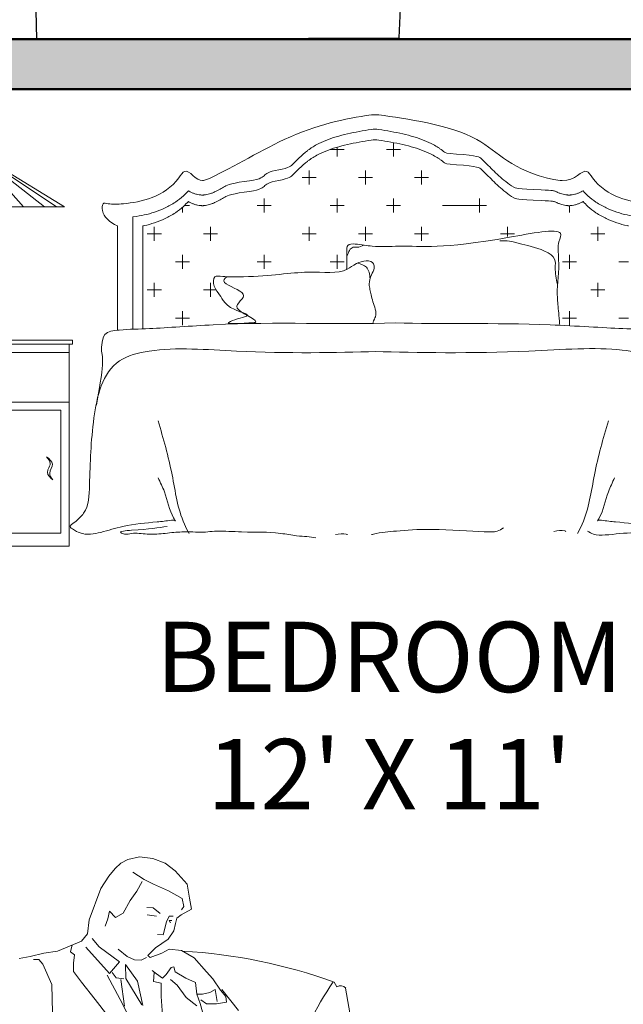
# Model space of a CAD drawing. Units: inches. Extents: x 1771 to 3025, y 319 to 889.
# Tile 28 of 35: x 2921 to 2982, y 521 to 619. Entities that reach past the tile are written whole.
import ezdxf

# ---------------------------------------------------------------- set-up
doc = ezdxf.new("R2010")
doc.units = ezdxf.units.IN
doc.header["$MEASUREMENT"] = 0
for name, color, linetype, lineweight in [('A-AREA-IDEN', 241, 'Continuous', 25), ('A-DOOR', 4, 'Continuous', 25), ('A-FURN', 8, 'Continuous', 18), ('A-WALL', 7, 'Continuous', 50), ('A-WALL-PATT', 254, 'Continuous', 13)]:
    doc.layers.add(name, color=color, linetype=linetype, lineweight=lineweight)
doc.styles.get("Standard").update_dxf_attribs({"font": 'arial.ttf'})

# ---------------------------------------------------------------- blocks, each defined once
blk = doc.blocks.new('A$C3908634B')
at = {"ltscale": 5}
for p, q in [((1200.2, 1046.3), (1218.1, 1046.3)), ((1176, 731), (1176, 731.7))]:
    blk.add_line(p, q, dxfattribs=at)
for p, q in [((1100.9, 962.2), (1134.6, 962.2)), ((1117.6, 945.1), (1117.6, 967.5)), ((1236.9, 962.2), (1271, 962.2)), ((1253.9, 945.1), (1253.9, 978.5)), ((266, 923.4), (356.4, 823.1)), ((278.7, 923.4), (406.8, 823.1)), ((284.7, 923.4), (436.3, 823.1)), ((290.6, 923.4), (456, 823.1)), ((1049.4, 876.9), (1049.4, 911)), ((1185.7, 876.9), (1185.7, 911)), ((1322.1, 876.9), (1322.1, 911)), ((1032.3, 894), (1066.4, 894)), ((1168.7, 894), (1202.8, 894)), ((1305.1, 894), (1339.1, 894)), ((940, 808.8), (940, 842.9)), ((1117.6, 808.8), (1117.6, 842.9)), ((1253.9, 808.8), (1253.9, 842.9)), ((1462.5, 808.8), (1462.5, 842.9)), ((237.5, 823.1), (456, 823.1)), ((741.7, 808.8), (741.7, 821.7)), ((746.2, 825.8), (758.8, 825.8)), ((922.9, 825.8), (957, 825.8)), ((1100.5, 825.8), (1134.6, 825.8)), ((1236.9, 825.8), (1271, 825.8)), ((1373.2, 825.8), (1479.5, 825.8)), ((1681.3, 808.8), (1681.3, 825.6)), ((621.3, 798.8), (621.3, 526)), ((645.8, 776.5), (645.8, 527)), ((673.5, 740.6), (673.5, 774.7)), ((809.9, 740.6), (809.9, 774.7)), ((1049.4, 740.6), (1049.4, 774.7)), ((1185.7, 740.6), (1185.7, 774.7)), ((1322.1, 740.6), (1322.1, 774.7)), ((1530.6, 751.3), (1530.6, 774.7)), ((1749.5, 740.6), (1749.5, 774.7)), ((656.5, 757.6), (690.6, 757.6)), ((792.9, 757.6), (827, 757.6)), ((1032.3, 757.6), (1066.4, 757.6)), ((1168.7, 757.6), (1202.8, 757.6)), ((1305.1, 757.6), (1339.1, 757.6)), ((1513.6, 757.6), (1547.7, 757.6)), ((1732.4, 757.6), (1766.5, 757.6)), ((741.7, 672.4), (741.7, 706.5)), ((940, 672.4), (940, 706.5)), ((1117.6, 672.4), (1117.6, 706.5)), ((1681.3, 672.4), (1681.3, 706.5)), ((724.7, 689.4), (758.8, 689.4)), ((922.9, 689.4), (957, 689.4)), ((1100.5, 689.4), (1134.6, 689.4)), ((1664.3, 689.4), (1698.3, 689.4)), ((1800.6, 689.4), (1824, 689.4)), ((656.5, 621.3), (690.6, 621.3)), ((673.5, 604.2), (673.5, 638.3)), ((792.9, 621.3), (823.2, 621.3)), ((809.9, 604.2), (809.9, 638.3)), ((1732.4, 621.3), (1766.5, 621.3)), ((1749.5, 604.2), (1749.5, 638.3)), ((724.7, 553.1), (758.8, 553.1)), ((741.7, 536), (741.7, 570.1)), ((1664.3, 553.1), (1698.3, 553.1)), ((1681.3, 536), (1681.3, 570.1)), ((1800.6, 553.1), (1824, 553.1)), ((475, 499.5), (0, 499.5)), ((475, 489.5), (0, 489.5)), ((467.1, 0), (467.1, 489.5)), ((475, 499.5), (475, 489.5)), ((467.1, 469.5), (8.7, 469.5)), ((467.1, 349.5), (8.7, 349.5)), ((447.1, 329.5), (28.7, 329.5)), ((447.1, 31.6), (447.1, 329.5)), ((467.1, 281.6), (467.1, 301.6)), ((28.7, 31.6), (447.1, 31.6)), ((8.7, 0), (467.1, 0))]:
    blk.add_line(p, q)
at = {"ltscale": 20}
blk.add_line((584.4, 776.7), (584.4, 523.7), dxfattribs=at)
for centre in [(1209.1, 956.2), (1209.1, 930.3)]:
    blk.add_arc(centre, 55.2, 80.5605, 99.4395)
for points in [[(584.4, 776.7), (563.9, 786.2), (546, 802.1), (547.3, 834.8), (564.5, 828.3), (620.6, 830.4), (706.4, 847.2), (752.1, 924.2), (778.1, 880.4), (846.1, 907.1), (1017.7, 1014.1), (1134.5, 1035.5), (1200.2, 1046.3)], [(1885.4, 776.7), (1905.9, 786.2), (1923.9, 802.1), (1922.5, 834.8), (1905.3, 828.3), (1849.2, 830.4), (1763.4, 847.2), (1717.7, 924.2), (1691.7, 880.4), (1541.2, 907.1), (1472.8, 1014.1), (1283.8, 1035.5), (1218.1, 1046.3)]]:
    blk.add_open_spline(points, degree=3, knots=[12.417853, 12.417853, 12.417853, 12.417853, 68.394536, 90.665986, 114.156853, 157.554067, 281.869614, 298.858744, 338.737111, 347.060176, 470.423438, 625.498764, 625.498764, 625.498764, 625.498764], dxfattribs=at)
for points, knots in [([(756.1, 861.8), (756.9, 861.3), (757.6, 860.9), (759.9, 859.6), (761.6, 858.7), (765.5, 856.8), (767.8, 855.8), (772.7, 854.1), (775.4, 853.3), (780.8, 852.2), (783.3, 851.8), (787.1, 851.6), (788.2, 851.5), (789.9, 851.5), (790.6, 851.5), (791.9, 851.5), (792.5, 851.5), (793.6, 851.6), (794.1, 851.6), (795.8, 851.8), (796.8, 851.9), (800.3, 852.3), (802.5, 852.8), (806.5, 853.8), (808.3, 854.3), (811.5, 855.4), (812.9, 855.9), (815.3, 856.9), (816.4, 857.4), (817.6, 857.9), (817.8, 858), (818.4, 858.2), (818.7, 858.4), (819.5, 858.7), (820, 859), (821.6, 859.7), (822.7, 860.2), (825.8, 861.7), (827.9, 862.8), (834, 866), (837.9, 868.3), (848.5, 874.9), (854.9, 879.4), (928.8, 888.8), (934.4, 893.5), (945, 903.2), (950, 908), (1000.9, 917.4), (1005.5, 922.1), (1014.4, 931), (1018.7, 935.3), (1027, 943.5), (1031.1, 947.3), (1036.9, 952.4), (1038.8, 954), (1042, 956.7), (1043.5, 957.9), (1045.8, 959.7), (1046.7, 960.3), (1048.5, 961.7), (1049.4, 962.3), (1052.1, 964.2), (1054, 965.5), (1059.7, 969.2), (1063.6, 971.5), (1074.8, 977.5), (1082.2, 980.9), (1098, 987.2), (1106.3, 990), (1123.7, 995.2), (1132.8, 997.5), (1151.5, 1001.8), (1161.1, 1003.8), (1180.5, 1007.4), (1190.2, 1009), (1200.1, 1010.7)], [328.6705, 328.6705, 328.6705, 328.6705, 329.609368, 329.609368, 331.487103, 331.487103, 333.620342, 333.620342, 335.753581, 335.753581, 337.507866, 337.507866, 338.182373, 338.182373, 338.607397, 338.607397, 338.959312, 338.959312, 339.311227, 339.311227, 340.015058, 340.015058, 341.722742, 341.722742, 343.430427, 343.430427, 345.138111, 345.138111, 346.845796, 346.845796, 347.37881, 347.37881, 347.911824, 347.911824, 348.977853, 348.977853, 351.109909, 351.109909, 355.374023, 355.374023, 363.902249, 363.902249, 379.258481, 379.258481, 394.614712, 394.614712, 409.970944, 409.970944, 425.327175, 425.327175, 440.683406, 440.683406, 456.039638, 456.039638, 463.285514, 463.285514, 469.01116, 469.01116, 472.593, 472.593, 476.17484, 476.17484, 483.338521, 483.338521, 497.665882, 497.665882, 522.309302, 522.309302, 546.952723, 546.952723, 571.596143, 571.596143, 596.239564, 596.239564, 619.876409, 619.876409, 619.876409, 619.876409]), ([(1713.7, 861.8), (1713, 861.3), (1712.2, 860.9), (1709.9, 859.6), (1708.2, 858.7), (1704.3, 856.8), (1702.1, 855.8), (1697.1, 854.1), (1694.4, 853.3), (1689.1, 852.2), (1686.5, 851.8), (1682.7, 851.6), (1681.7, 851.5), (1679.9, 851.5), (1679.2, 851.5), (1678, 851.5), (1677.4, 851.5), (1676.2, 851.6), (1675.7, 851.6), (1674.1, 851.8), (1673, 851.9), (1669.5, 852.3), (1667.3, 852.8), (1663.3, 853.8), (1661.5, 854.3), (1658.4, 855.4), (1657, 855.9), (1654.5, 856.9), (1653.4, 857.4), (1652.2, 857.9), (1652, 858), (1651.4, 858.2), (1651.2, 858.4), (1650.4, 858.7), (1649.8, 859), (1648.2, 859.7), (1647.1, 860.2), (1644, 861.7), (1641.9, 862.8), (1553.3, 866), (1549.4, 868.3), (1538.8, 874.9), (1532.4, 879.4), (1520.4, 888.8), (1514.8, 893.5), (1504.2, 903.2), (1499.2, 908), (1489.5, 917.4), (1484.9, 922.1), (1476.1, 931), (1471.8, 935.3), (1463.4, 943.5), (1459.4, 947.3), (1381.4, 952.4), (1379.5, 954), (1376.2, 956.7), (1374.8, 957.9), (1372.5, 959.7), (1371.6, 960.3), (1369.8, 961.7), (1368.9, 962.3), (1366.2, 964.2), (1364.3, 965.5), (1358.6, 969.2), (1354.6, 971.5), (1343.5, 977.5), (1336, 980.9), (1320.2, 987.2), (1311.9, 990), (1294.6, 995.2), (1285.5, 997.5), (1266.8, 1001.8), (1257.2, 1003.8), (1237.8, 1007.4), (1228.1, 1009), (1218.2, 1010.7)], [328.6705, 328.6705, 328.6705, 328.6705, 329.609368, 329.609368, 331.487103, 331.487103, 333.620342, 333.620342, 335.753581, 335.753581, 337.507866, 337.507866, 338.182373, 338.182373, 338.607397, 338.607397, 338.959312, 338.959312, 339.311227, 339.311227, 340.015058, 340.015058, 341.722742, 341.722742, 343.430427, 343.430427, 345.138111, 345.138111, 346.845796, 346.845796, 347.37881, 347.37881, 347.911824, 347.911824, 348.977853, 348.977853, 351.109909, 351.109909, 355.374023, 355.374023, 363.902249, 363.902249, 379.258481, 379.258481, 394.614712, 394.614712, 409.970943, 409.970943, 425.327175, 425.327175, 440.683406, 440.683406, 456.039637, 456.039637, 463.285514, 463.285514, 469.011154, 469.011154, 472.592992, 472.592992, 476.17483, 476.17483, 483.338506, 483.338506, 497.665857, 497.665857, 522.309275, 522.309275, 546.952693, 546.952693, 571.59611, 571.59611, 596.239528, 596.239528, 619.876409, 619.876409, 619.876409, 619.876409]), ([(756.1, 835.9), (756.9, 835.5), (757.6, 835), (759.9, 833.7), (761.6, 832.8), (765.5, 830.9), (767.8, 830), (772.7, 828.2), (775.4, 827.5), (780.8, 826.3), (783.3, 826), (787.1, 825.7), (788.2, 825.7), (789.9, 825.6), (790.6, 825.6), (791.9, 825.6), (792.5, 825.7), (793.6, 825.7), (794.1, 825.8), (795.8, 825.9), (796.8, 826), (800.3, 826.5), (802.5, 826.9), (806.5, 827.9), (808.3, 828.5), (811.5, 829.5), (812.9, 830.1), (815.3, 831), (816.4, 831.5), (817.6, 832), (817.8, 832.1), (818.4, 832.4), (818.7, 832.5), (819.5, 832.9), (820, 833.1), (821.6, 833.8), (822.7, 834.3), (825.8, 835.9), (827.9, 836.9), (834, 840.2), (837.9, 842.4), (848.5, 849), (854.9, 853.6), (928.8, 862.9), (934.4, 867.7), (945, 877.3), (950, 882.1), (1000.9, 891.6), (1005.5, 896.2), (1014.4, 905.2), (1018.7, 909.5), (1027, 917.6), (1031.1, 921.4), (1036.9, 926.6), (1038.8, 928.2), (1042, 930.9), (1043.5, 932), (1045.8, 933.8), (1046.7, 934.5), (1048.5, 935.8), (1049.4, 936.4), (1052.1, 938.4), (1054, 939.6), (1059.7, 943.3), (1063.6, 945.6), (1074.8, 951.6), (1082.2, 955), (1098, 961.3), (1106.3, 964.2), (1123.7, 969.3), (1132.8, 971.6), (1151.5, 975.9), (1161.1, 977.9), (1180.5, 981.5), (1190.2, 983.2), (1200.1, 984.8)], [328.6705, 328.6705, 328.6705, 328.6705, 329.609368, 329.609368, 331.487103, 331.487103, 333.620342, 333.620342, 335.753581, 335.753581, 337.507866, 337.507866, 338.182373, 338.182373, 338.607397, 338.607397, 338.959312, 338.959312, 339.311227, 339.311227, 340.015058, 340.015058, 341.722742, 341.722742, 343.430427, 343.430427, 345.138111, 345.138111, 346.845796, 346.845796, 347.37881, 347.37881, 347.911824, 347.911824, 348.977853, 348.977853, 351.109909, 351.109909, 355.374023, 355.374023, 363.902249, 363.902249, 379.258481, 379.258481, 394.614712, 394.614712, 409.970944, 409.970944, 425.327175, 425.327175, 440.683406, 440.683406, 456.039638, 456.039638, 463.285514, 463.285514, 469.01116, 469.01116, 472.593, 472.593, 476.17484, 476.17484, 483.338521, 483.338521, 497.665882, 497.665882, 522.309302, 522.309302, 546.952723, 546.952723, 571.596143, 571.596143, 596.239564, 596.239564, 619.876409, 619.876409, 619.876409, 619.876409]), ([(1713.7, 835.9), (1713, 835.5), (1712.2, 835), (1709.9, 833.7), (1708.2, 832.8), (1704.3, 830.9), (1702.1, 830), (1697.1, 828.2), (1694.4, 827.5), (1689.1, 826.3), (1686.5, 826), (1682.7, 825.7), (1681.7, 825.7), (1679.9, 825.6), (1679.2, 825.6), (1678, 825.6), (1677.4, 825.7), (1676.2, 825.7), (1675.7, 825.8), (1674.1, 825.9), (1673, 826), (1669.5, 826.5), (1667.3, 826.9), (1663.3, 827.9), (1661.5, 828.5), (1658.4, 829.5), (1657, 830.1), (1654.5, 831), (1653.4, 831.5), (1652.2, 832), (1652, 832.1), (1651.4, 832.4), (1651.2, 832.5), (1650.4, 832.9), (1649.8, 833.1), (1648.2, 833.8), (1647.1, 834.3), (1644, 835.9), (1641.9, 836.9), (1553.3, 840.2), (1549.4, 842.4), (1538.8, 849), (1532.4, 853.6), (1520.4, 862.9), (1514.8, 867.7), (1504.2, 877.3), (1499.2, 882.1), (1489.5, 891.6), (1484.9, 896.2), (1476.1, 905.2), (1471.8, 909.5), (1463.4, 917.6), (1459.4, 921.4), (1381.4, 926.6), (1379.5, 928.2), (1376.2, 930.9), (1374.8, 932), (1372.5, 933.8), (1371.6, 934.5), (1369.8, 935.8), (1368.9, 936.4), (1366.2, 938.4), (1364.3, 939.6), (1358.6, 943.3), (1354.6, 945.6), (1343.5, 951.6), (1336, 955), (1320.2, 961.3), (1311.9, 964.2), (1294.6, 969.3), (1285.5, 971.6), (1266.8, 975.9), (1257.2, 977.9), (1237.8, 981.5), (1228.1, 983.2), (1218.2, 984.8)], [328.6705, 328.6705, 328.6705, 328.6705, 329.609368, 329.609368, 331.487103, 331.487103, 333.620342, 333.620342, 335.753581, 335.753581, 337.507866, 337.507866, 338.182373, 338.182373, 338.607397, 338.607397, 338.959312, 338.959312, 339.311227, 339.311227, 340.015058, 340.015058, 341.722742, 341.722742, 343.430427, 343.430427, 345.138111, 345.138111, 346.845796, 346.845796, 347.37881, 347.37881, 347.911824, 347.911824, 348.977853, 348.977853, 351.109909, 351.109909, 355.374023, 355.374023, 363.902249, 363.902249, 379.258481, 379.258481, 394.614712, 394.614712, 409.970943, 409.970943, 425.327175, 425.327175, 440.683406, 440.683406, 456.039637, 456.039637, 463.285514, 463.285514, 469.011154, 469.011154, 472.592992, 472.592992, 476.17483, 476.17483, 483.338506, 483.338506, 497.665857, 497.665857, 522.309275, 522.309275, 546.952693, 546.952693, 571.59611, 571.59611, 596.239528, 596.239528, 619.876409, 619.876409, 619.876409, 619.876409]), ([(621.3, 798.8), (633.4, 799.9), (641.2, 801.3), (657.3, 805), (665.7, 807.2), (682.6, 812.8), (691.1, 816.1), (708.1, 824.2), (716.5, 828.9), (731.3, 839), (737.9, 844.1), (748.3, 853.5), (752.3, 857.5), (756.1, 861.8)], [179.330708, 179.330708, 179.330708, 179.330708, 196.086144, 196.086144, 213.445516, 213.445516, 230.804888, 230.804888, 248.16426, 248.16426, 262.451931, 262.451931, 271.832526, 271.832526, 271.832526, 271.832526]), ([(1848.6, 798.8), (1836.4, 799.9), (1828.6, 801.3), (1812.5, 805), (1804.1, 807.2), (1787.2, 812.8), (1778.7, 816.1), (1761.8, 824.2), (1753.4, 828.9), (1738.5, 839), (1731.9, 844.1), (1721.5, 853.5), (1717.5, 857.5), (1713.7, 861.8)], [179.400376, 179.400376, 179.400376, 179.400376, 196.086144, 196.086144, 213.445516, 213.445516, 230.804888, 230.804888, 248.16426, 248.16426, 262.451931, 262.451931, 271.832526, 271.832526, 271.832526, 271.832526]), ([(645.8, 776.5), (646.9, 776.7), (648, 777), (657.3, 779.1), (665.7, 781.3), (682.6, 786.9), (691.1, 790.3), (708.1, 798.3), (716.5, 803), (731.3, 813.1), (737.9, 818.2), (748.3, 827.7), (752.3, 831.7), (756.1, 835.9)], [193.740688, 193.740688, 193.740688, 193.740688, 196.086144, 196.086144, 213.445516, 213.445516, 230.804888, 230.804888, 248.16426, 248.16426, 262.451931, 262.451931, 271.832526, 271.832526, 271.832526, 271.832526]), ([(1824, 776.5), (1822.9, 776.7), (1821.8, 777), (1812.5, 779.1), (1804.1, 781.3), (1787.2, 786.9), (1778.7, 790.3), (1761.8, 798.3), (1753.4, 803), (1738.5, 813.1), (1731.9, 818.2), (1721.5, 827.7), (1717.5, 831.7), (1713.7, 835.9)], [193.740688, 193.740688, 193.740688, 193.740688, 196.086144, 196.086144, 213.445516, 213.445516, 230.804888, 230.804888, 248.16426, 248.16426, 262.451931, 262.451931, 271.832526, 271.832526, 271.832526, 271.832526]), ([(1512.2, 740.7), (1519.9, 740.7), (1533.1, 740.8), (1553.9, 735.5), (1652.4, 710.7), (1643.1, 675.3), (1648.8, 648.1), (1651.8, 634.5), (1651.9, 634)], [0, 0, 0, 0, 31.268494, 53.71641, 83.24833, 138.583941, 192.96698, 194.695488, 194.695488, 194.695488, 194.695488]), ([(1181.8, 730.2), (1176.9, 727.3), (1167.9, 723.5), (1152.3, 726.4), (1145.2, 713.6), (1142.1, 705.5), (1140.6, 701.2)], [16.588235, 16.588235, 16.588235, 16.588235, 39.368234, 56.465167, 72.647278, 91.317886, 91.317886, 91.317886, 91.317886]), ([(1167.2, 686.5), (1175.5, 684.3), (1192.8, 677.8), (1196.3, 659.6), (1197.1, 648.3)], [13.535772, 13.535772, 13.535772, 13.535772, 45.871957, 87.312392, 87.312392, 87.312392, 87.312392]), ([(849.2, 653.1), (844.3, 648.8), (832.7, 636.7), (919.4, 609.9), (841.8, 577.9), (927.1, 550.1), (918.1, 541), (854.7, 539.8)], [5.952535, 5.952535, 5.952535, 5.952535, 29.258845, 70.114919, 115.518645, 162.322231, 169.813565, 169.813565, 169.813565, 169.813565]), ([(412.3, 216.6), (419.2, 211), (432.8, 199.9), (414.9, 178.1), (423.4, 166), (427.2, 160.5)], [0, 0, 0, 0, 22.772447, 45.052082, 63.466582, 63.466582, 63.466582, 63.466582]), ([(412.3, 216.6), (416.7, 211.4), (424.6, 201.9), (416.9, 189), (411.8, 174.1), (420.6, 166.3), (427.2, 160.5)], [0, 0, 0, 0, 18.381528, 32.980054, 40.875646, 63.595153, 63.595153, 63.595153, 63.595153])]:
    blk.add_open_spline(points, degree=3, knots=knots)
at = {"ltscale": 5}
for points, knots in [([(1140.2, 671), (1140.5, 684.2), (1141, 702.6), (1139.6, 733.3), (1171.5, 732.8), (1207.8, 724.4), (1313, 731.7), (1377.9, 716.1), (1675.3, 776), (1653.6, 739.3), (1653.4, 708.6), (1656.7, 669.4), (1649.8, 624.8), (1652.8, 584.9), (1655.4, 559.2), (1656.8, 538.3)], [3.603347, 3.603347, 3.603347, 3.603347, 60.838375, 82.182907, 107.012175, 163.177093, 249.239778, 501.114283, 577.787612, 607.274607, 630.949286, 706.159707, 762.92633, 812.910096, 867.096105, 867.096105, 867.096105, 867.096105]), ([(853.1, 539.8), (853.8, 547.4), (919.3, 558.2), (845.3, 575.8), (836.7, 609.7), (818, 623.2), (814.4, 657.6), (840.5, 653), (943.6, 652.6), (1051.1, 671.7), (1127.7, 657.4), (1165, 689.4), (1205, 697), (1208.2, 671.1), (1198.6, 657.5), (1193.8, 634.4), (1197.9, 619.2), (1201.2, 597.1), (1215.4, 563.6), (1206.8, 549.2), (1203.5, 540.2)], [33.020195, 33.020195, 33.020195, 33.020195, 57.294753, 90.473933, 194.149416, 257.058105, 304.592565, 338.383824, 389.043604, 577.649845, 759.359611, 813.032269, 898.973184, 920.659088, 956.429806, 1000.911745, 1042.797508, 1121.842246, 1191.460876, 1213.109701, 1213.109701, 1213.109701, 1213.109701]), ([(533.2, 342.2), (554.6, 456.3), (543.3, 464.8), (546.8, 491.4), (549.9, 520.4), (602.8, 525.9), (675.3, 527.2), (929.2, 547.1), (1113.3, 536.9), (1259.7, 541.4)], [0, 0, 0, 0, 32.681627, 48.455722, 75.25348, 112.004017, 183.381957, 310.642358, 688.088714, 688.088714, 688.088714, 688.088714]), ([(1911, 390.4), (1911.9, 458.8), (1930, 464.8), (1926.5, 491.4), (1923.4, 520.4), (1870.5, 525.9), (1798, 527.2), (1556.5, 543.7), (1364.8, 538.4), (1259.7, 541.4)], [0, 0, 0, 0, 32.681627, 48.455722, 75.25348, 112.004017, 183.381957, 310.642358, 588.939547, 588.939547, 588.939547, 588.939547]), ([(482.8, 59.4), (489.8, 65.8), (514.7, 88.6), (517.4, 182.5), (520.5, 297.5), (551.9, 447.1), (697, 485.5), (926.3, 465.8), (1116.6, 468.9), (1210.9, 472.2)], [0, 0, 0, 0, 28.320233, 100.953775, 269.820348, 420.691469, 489.161544, 656.134073, 940.569207, 940.569207, 940.569207, 940.569207]), ([(1990.5, 59.4), (1983.5, 65.8), (1958.6, 88.6), (1942.6, 182.5), (1920.4, 297.5), (1912.1, 455.6), (1776.3, 485.5), (1526.4, 465.8), (1305.2, 468.9), (1210.9, 472.2)], [0, 0, 0, 0, 28.320233, 100.953775, 269.820348, 420.691469, 489.161544, 656.134073, 940.569207, 940.569207, 940.569207, 940.569207]), ([(682.9, 304.1), (695.4, 260.8), (719.1, 178.1), (730.8, 82.2), (753.9, 38.3), (757.8, 30.9)], [0, 0, 0, 0, 135.247847, 258.692787, 283.800228, 283.800228, 283.800228, 283.800228]), ([(1775.2, 304.1), (1762.7, 260.8), (1739, 178.1), (1727.3, 82.2), (1704.2, 38.3), (1700.3, 30.9)], [0, 0, 0, 0, 135.247847, 258.692787, 283.800228, 283.800228, 283.800228, 283.800228]), ([(682.9, 165.6), (688.3, 154.5), (703.5, 123.2), (710.2, 85), (723.1, 63.5), (724.6, 61.1)], [0, 0, 0, 0, 37.234018, 105.386078, 113.844905, 113.844905, 113.844905, 113.844905]), ([(1790.4, 165.6), (1785, 154.5), (1769.8, 123.2), (1763.1, 85), (1750.2, 63.5), (1748.7, 61.1)], [0, 0, 0, 0, 37.234018, 105.386078, 113.844905, 113.844905, 113.844905, 113.844905]), ([(482.8, 59.4), (474.7, 54.3), (464, 47.4), (477.3, 41.4), (486.1, 33.4), (496.5, 31.3), (502.9, 30)], [0, 0, 0, 0, 19.035414, 25.269998, 36.960672, 56.00812, 56.00812, 56.00812, 56.00812]), ([(504.2, 28.9), (509, 28.7), (522.4, 28.3), (553.7, 35.4), (605.7, 52.4), (665.1, 57), (705.3, 61.4), (721.5, 63.6), (724.2, 61.4), (724.6, 61.1)], [0, 0, 0, 0, 14.447875, 40.468341, 96.220884, 181.018327, 216.046098, 224.609189, 226.185962, 226.185962, 226.185962, 226.185962]), ([(1969.1, 28.9), (1964.3, 28.7), (1950.9, 28.3), (1919.6, 35.4), (1867.6, 52.4), (1808.2, 57), (1768, 61.4), (1751.8, 63.6), (1749.1, 61.4), (1748.7, 61.1)], [0, 0, 0, 0, 14.447875, 40.468341, 96.220884, 181.018327, 216.046098, 224.609189, 226.185962, 226.185962, 226.185962, 226.185962]), ([(704.5, 47.7), (683.7, 44.6), (656.6, 40.6), (582.3, 36), (604.8, 26.7), (618.5, 32.3), (643.5, 30.4), (675.7, 27.4), (715, 33.3), (758.1, 35.6), (793.8, 32.4), (824.3, 37.8), (918.5, 32.1), (952.2, 36.4), (1023, 23.8), (1044.1, 24.1), (1058.3, 21.3), (1065.7, 20.4)], [0, 0, 0, 0, 87.513803, 114.592793, 124.77702, 141.903576, 160.817021, 198.691115, 240.471478, 280.23486, 329.410006, 348.41762, 373.077233, 428.05708, 447.802257, 468.691939, 491.310217, 491.310217, 491.310217, 491.310217]), ([(1113.3, 28), (1122.2, 29.4), (1132.2, 31.9), (1141.4, 28.4), (1142.4, 28)], [516.212662, 516.212662, 516.212662, 516.212662, 542.681017, 546.007116, 546.007116, 546.007116, 546.007116]), ([(1200.5, 28), (1202, 28.4), (1222.7, 33.5), (1266.3, 36.8), (1334.2, 43.2), (1462.5, 35), (1502.7, 33.5), (1515.8, 41.2), (1520.7, 44.1)], [590.079786, 590.079786, 590.079786, 590.079786, 594.646549, 651.888327, 725.747367, 797.841373, 826.274406, 843.189267, 843.189267, 843.189267, 843.189267]), ([(1643.2, 35.6), (1652.1, 37), (1662.2, 39.5), (1671.4, 36), (1672.4, 35.6)], [516.212662, 516.212662, 516.212662, 516.212662, 542.681017, 546.007116, 546.007116, 546.007116, 546.007116]), ([(1972.3, 20.4), (1970.7, 20.8), (1950, 25.9), (1906.5, 29.2), (1838.6, 35.6), (1782.4, 27.4), (1742.2, 25.9), (1729.1, 33.6), (1724.3, 36.5)], [590.079786, 590.079786, 590.079786, 590.079786, 594.646549, 651.888327, 725.747367, 797.841373, 826.274406, 843.189267, 843.189267, 843.189267, 843.189267])]:
    blk.add_open_spline(points, degree=3, knots=knots, dxfattribs=at)
blk = doc.blocks.new('A$C0DCF6C46')
for p, q in [((1202.6, 1072.4), (1213.4, 1083.3)), ((1202.6, 1072.4), (1213.4, 1083.3)), ((1213.4, 1083.3), (1227.6, 1090.4)), ((1213.4, 1083.3), (1227.6, 1090.4)), ((1227.6, 1090.4), (1251, 1095.4)), ((1227.6, 1090.4), (1251, 1095.4)), ((1251, 1095.4), (1277.5, 1092)), ((1251, 1095.4), (1277.5, 1092)), ((1277.5, 1092), (1301.8, 1082.8)), ((1277.5, 1092), (1301.8, 1082.8)), ((1301.8, 1082.8), (1321.9, 1067.8)), ((1301.8, 1082.8), (1321.9, 1067.8)), ((1173.6, 1032.9), (1189.7, 1057.2)), ((1173.6, 1032.9), (1189.7, 1057.2)), ((1189.7, 1057.2), (1202.6, 1072.4)), ((1189.7, 1057.2), (1202.6, 1072.4)), ((1259.7, 1050.3), (1237.5, 1065.3)), ((1259.7, 1050.3), (1237.5, 1065.3)), ((1321.9, 1067.8), (1345.5, 1041.1)), ((1321.9, 1067.8), (1345.5, 1041.1)), ((1255.9, 1046.6), (1245.7, 1027.6)), ((1255.9, 1046.6), (1245.7, 1027.6)), ((1278.7, 1041.6), (1259.7, 1050.3)), ((1278.7, 1041.6), (1259.7, 1050.3)), ((1308.3, 1028.1), (1278.7, 1041.6)), ((1308.3, 1028.1), (1278.7, 1041.6)), ((1345.5, 1041.1), (1350.1, 1013.5)), ((1345.5, 1041.1), (1350.1, 1013.5)), ((1150.8, 970.5), (1173.6, 1032.9)), ((1150.8, 970.5), (1173.6, 1032.9)), ((1245.7, 1027.6), (1232.3, 1009.1)), ((1245.7, 1027.6), (1232.3, 1009.1)), ((1335.8, 1012.5), (1308.3, 1028.1)), ((1335.8, 1012.5), (1308.3, 1028.1)), ((1232.3, 1009.1), (1218.3, 983.7)), ((1232.3, 1009.1), (1218.3, 983.7)), ((1338.8, 997.1), (1335.8, 1012.5)), ((1338.8, 997.1), (1335.8, 1012.5)), ((1350.1, 1013.5), (1354.2, 991.7)), ((1350.1, 1013.5), (1354.2, 991.7)), ((1190.8, 987.7), (1188, 972.3)), ((1190.8, 987.7), (1188, 972.3)), ((1202.9, 975.4), (1190.8, 987.7)), ((1202.9, 975.4), (1190.8, 987.7)), ((1218.3, 983.7), (1202.9, 975.4)), ((1218.3, 983.7), (1202.9, 975.4)), ((1277.8, 994.4), (1265.6, 995)), ((1277.8, 994.4), (1265.6, 995)), ((1266, 980.7), (1284.6, 977.9)), ((1266, 980.7), (1284.6, 977.9)), ((1291.5, 983.2), (1277.8, 994.4)), ((1291.5, 983.2), (1277.8, 994.4)), ((1333.4, 980.2), (1324.9, 973.9)), ((1333.4, 980.2), (1324.9, 973.9)), ((1354.2, 991.7), (1333.4, 980.2)), ((1354.2, 991.7), (1333.4, 980.2)), ((1334, 990.3), (1338.8, 997.1)), ((1334, 990.3), (1338.8, 997.1)), ((1147.4, 942.9), (1150.8, 970.5)), ((1147.4, 942.9), (1150.8, 970.5)), ((1188, 972.3), (1182.6, 958)), ((1188, 972.3), (1182.6, 958)), ((1304.1, 966.6), (1297.6, 940.6)), ((1304.1, 966.6), (1297.6, 940.6)), ((1309.5, 977.7), (1304.1, 966.6)), ((1309.5, 977.7), (1304.1, 966.6)), ((1309.4, 969), (1312.6, 964.7)), ((1314.7, 968.9), (1309.4, 969)), ((1309.4, 969), (1312.6, 964.7)), ((1314.7, 968.9), (1309.4, 969)), ((1317.5, 977.7), (1309.5, 977.7)), ((1317.5, 977.7), (1309.5, 977.7)), ((1322.1, 963.3), (1318.8, 948.5)), ((1322.1, 963.3), (1318.8, 948.5)), ((1324.9, 973.9), (1322.1, 963.3)), ((1324.9, 973.9), (1322.1, 963.3)), ((1135.7, 928.2), (1147.4, 942.9)), ((1135.7, 928.2), (1147.4, 942.9)), ((1297.6, 940.6), (1286.8, 941.4)), ((1297.6, 940.6), (1286.8, 941.4)), ((1318.8, 948.5), (1307.6, 932.1)), ((1318.8, 948.5), (1307.6, 932.1)), ((1087.8, 908.4), (1135.7, 928.2)), ((1087.8, 908.4), (1135.7, 928.2)), ((1117, 920.9), (1113.7, 907.1)), ((1117, 920.9), (1113.7, 907.1)), ((1170.4, 917.1), (1156.8, 933.1)), ((1170.4, 917.1), (1156.8, 933.1)), ((1307.6, 932.1), (1282.5, 914.8)), ((1307.6, 932.1), (1282.5, 914.8)), ((1033.6, 897.7), (1060.7, 904.4)), ((1033.6, 897.7), (1060.7, 904.4)), ((1060.7, 904.4), (1087.8, 908.4)), ((1060.7, 904.4), (1087.8, 908.4)), ((1113.7, 907.1), (1121.7, 900.7)), ((1113.7, 907.1), (1121.7, 900.7)), ((1121.7, 900.7), (1119.4, 884.3)), ((1121.7, 900.7), (1119.4, 884.3)), ((1190.9, 864.1), (1144, 915.9)), ((1190.9, 864.1), (1144, 915.9)), ((1211.2, 886.7), (1170.4, 917.1)), ((1211.2, 886.7), (1170.4, 917.1)), ((1225.9, 897.6), (1208.3, 912.3)), ((1225.9, 897.6), (1208.3, 912.3)), ((1282.5, 914.8), (1267, 899.5)), ((1282.5, 914.8), (1267, 899.5)), ((1271.7, 895.8), (1295.1, 904.1)), ((1271.7, 895.8), (1295.1, 904.1)), ((1295.1, 904.1), (1310, 911.9)), ((1295.1, 904.1), (1310, 911.9)), ((1310, 911.9), (1334.4, 909.6)), ((1310, 911.9), (1334.4, 909.6)), ((1334.4, 909.6), (1359.2, 894.6)), ((1334.4, 909.6), (1359.2, 894.6)), ((1011.8, 893.6), (1033.6, 897.7)), ((1011.8, 893.6), (1033.6, 897.7)), ((1039.9, 891.8), (1050.5, 891.7)), ((1039.9, 891.8), (1050.5, 891.7)), ((1050.5, 891.7), (1058.4, 882.1)), ((1050.5, 891.7), (1058.4, 882.1)), ((1058.4, 882.1), (1076.1, 842.2)), ((1058.4, 882.1), (1076.1, 842.2)), ((1119.4, 884.3), (1119.3, 867.8)), ((1119.4, 884.3), (1119.3, 867.8)), ((1211.2, 886.7), (1190.9, 864.1)), ((1211.2, 886.7), (1190.9, 864.1)), ((1222.8, 881.9), (1223.6, 853.9)), ((1247, 848.8), (1222.8, 881.9)), ((1222.8, 881.9), (1223.6, 853.9)), ((1247, 848.8), (1222.8, 881.9)), ((1240.6, 890.8), (1225.9, 897.6)), ((1240.6, 890.8), (1225.9, 897.6)), ((1254.3, 890.2), (1240.6, 890.8)), ((1254.3, 890.2), (1240.6, 890.8)), ((1264.4, 895.9), (1254.3, 890.2)), ((1264.4, 895.9), (1254.3, 890.2)), ((1267, 899.5), (1271.7, 895.8)), ((1267, 899.5), (1271.7, 895.8)), ((1359.2, 894.6), (1384, 866.8)), ((1359.2, 894.6), (1384, 866.8)), ((1119.3, 867.8), (1135.5, 846.5)), ((1119.3, 867.8), (1135.5, 846.5)), ((1196.7, 865.6), (1204.6, 855)), ((1196.7, 865.6), (1204.6, 855)), ((1275.8, 869.8), (1284.7, 863.3)), ((1275.8, 869.8), (1284.7, 863.3)), ((1278.8, 848), (1280, 865.5)), ((1278.8, 848), (1280, 865.5)), ((1284.7, 863.3), (1296.3, 854.2)), ((1284.7, 863.3), (1296.3, 854.2)), ((1296.3, 854.2), (1303.8, 861.6)), ((1296.3, 854.2), (1303.8, 861.6)), ((1303.8, 861.6), (1313.5, 875.8)), ((1303.8, 861.6), (1313.5, 875.8)), ((1313.5, 875.8), (1318.8, 876.9)), ((1313.5, 875.8), (1318.8, 876.9)), ((1318.8, 876.9), (1321.4, 867.3)), ((1318.8, 876.9), (1321.4, 867.3)), ((1321.4, 867.3), (1342.5, 854.4)), ((1321.4, 867.3), (1342.5, 854.4)), ((1384, 866.8), (1396.6, 853.4)), ((1384, 866.8), (1396.6, 853.4)), ((1076.1, 842.2), (1077.8, 785.9)), ((1076.1, 842.2), (1077.8, 785.9)), ((1135.5, 846.5), (1162.3, 812.3)), ((1135.5, 846.5), (1162.3, 812.3)), ((1186.6, 860.4), (1212.2, 811.9)), ((1186.6, 860.4), (1212.2, 811.9)), ((1204.6, 855), (1219.4, 853.2)), ((1204.6, 855), (1219.4, 853.2)), ((1213.6, 851.7), (1221.1, 799.1)), ((1213.6, 851.7), (1221.1, 799.1)), ((1223.6, 853.9), (1255.4, 801.3)), ((1223.6, 853.9), (1255.4, 801.3)), ((1257.2, 799.9), (1247, 848.8)), ((1257.2, 799.9), (1247, 848.8)), ((1293.6, 844.7), (1278.8, 848)), ((1293.6, 844.7), (1278.8, 848)), ((1293.9, 818.2), (1293.6, 844.7)), ((1293.9, 818.2), (1293.6, 844.7)), ((1325.9, 840.7), (1312.2, 852)), ((1325.9, 840.7), (1312.2, 852)), ((1342.5, 854.4), (1362, 845.8)), ((1342.5, 854.4), (1362, 845.8)), ((1362, 845.8), (1365, 822.9)), ((1362, 845.8), (1365, 822.9)), ((1396.6, 853.4), (1411.8, 831)), ((1396.6, 853.4), (1411.8, 831)), ((1637.6, 846.8), (1643.1, 837.5)), ((1637.6, 846.8), (1643.1, 837.5)), ((1343.2, 816.2), (1325.9, 840.7)), ((1343.2, 816.2), (1325.9, 840.7)), ((1376.2, 822.8), (1365, 822.9)), ((1365, 822.9), (1371.3, 804.3)), ((1376.2, 822.8), (1365, 822.9)), ((1365, 822.9), (1371.3, 804.3)), ((1390.5, 825.9), (1376.2, 822.8)), ((1390.5, 825.9), (1376.2, 822.8)), ((1401.2, 832.2), (1390.5, 825.9)), ((1401.2, 832.2), (1390.5, 825.9)), ((1405.2, 808.3), (1401.2, 832.2)), ((1405.2, 808.3), (1401.2, 832.2)), ((1411.8, 831), (1422.3, 818.2)), ((1411.8, 831), (1422.3, 818.2)), ((1414.4, 832.1), (1447.5, 790.5)), ((1414.4, 832.1), (1447.5, 790.5)), ((1680.1, 723.7), (1660.3, 834.6)), ((1680.1, 723.7), (1660.3, 834.6)), ((1162.3, 812.3), (1187.5, 779.8)), ((1162.3, 812.3), (1187.5, 779.8)), ((1212.2, 811.9), (1236.7, 763.5)), ((1212.2, 811.9), (1236.7, 763.5)), ((1296.3, 781), (1293.9, 818.2)), ((1296.3, 781), (1293.9, 818.2)), ((1364.9, 799.6), (1343.2, 816.2)), ((1364.9, 799.6), (1343.2, 816.2)), ((1371.3, 804.3), (1380.5, 770.8)), ((1371.3, 804.3), (1380.5, 770.8)), ((1384, 803.7), (1372.4, 811.7)), ((1384, 803.7), (1372.4, 811.7)), ((1403.6, 803.5), (1384, 803.7)), ((1403.6, 803.5), (1384, 803.7)), ((1423.8, 807.1), (1403.6, 803.5)), ((1423.8, 807.1), (1403.6, 803.5)), ((1422.3, 818.2), (1423.8, 807.1)), ((1422.3, 818.2), (1423.8, 807.1))]:
    blk.add_line(p, q)
for centre, radius, start, end in [((1273.4, -169.1), 1079.2, 70.279, 86.636), ((1273.4, -169.1), 1079.2, 70.279, 86.636), ((2335, 385.5), 838.2, 146.5555, 159.4144), ((2335, 385.5), 838.2, 146.5555, 159.4144), ((1650.3, 825), 14.4, 42.1894, 120.2274), ((1650.3, 825), 14.4, 42.1894, 120.2274)]:
    blk.add_arc(centre, radius, start, end)
blk = doc.blocks.new('A$C4223307F')
blk.add_blockref('A$C0DCF6C46', (0, 0))
blk = doc.blocks.new('A$C061F63B6')
blk.add_blockref('A$C4223307F', (0, 0))
blk = doc.blocks.new('DOOR-35')
blk.add_lwpolyline([(35.881, 36.185), (32.957, 36.297), (33.165, 0), (36, 0.055)], close=True)
blk.add_arc((35.225, 1.111), 35.259, 93.68792, 177.49253)

msp = doc.modelspace()

# ---------------------------------------------------------------- hatches: boundary and pattern name
at = {"layer": 'A-WALL-PATT'}
h = msp.add_hatch(color=256, dxfattribs=at)
h.dxf.hatch_style = 1
h.paths.add_polyline_path([(2870.685, 879.484), (2892.728, 879.484), (2892.728, 889.484), (2842.685, 889.484), (2842.685, 879.484), (2865.685, 879.484), (2865.685, 831.484), (2870.685, 831.484)])
h.paths.add_polyline_path([(2983.637, 889.484), (2940.728, 889.484), (2940.728, 879.484), (2961.685, 879.484), (2961.685, 795.484), (2865.685, 795.484), (2865.685, 759.484), (2865.685, 665.484), (2870.685, 665.484), (2870.685, 712.85), (2870.685, 790.484), (2978.685, 790.484), (2978.685, 795.484), (2966.685, 795.484), (2966.685, 879.484), (2983.637, 879.484)])
h.paths.add_polyline_path([(3024.685, 889.484), (3001.637, 889.484), (3001.637, 879.484), (3014.685, 879.484), (3014.685, 790.484), (3014.685, 769.459), (3024.685, 769.459)])
h.paths.add_polyline_path([(3024.685, 721.459), (3014.685, 721.459), (3014.685, 670.484), (2906.685, 670.484), (2906.685, 665.484), (2925.685, 665.484), (2925.685, 653.484), (2930.685, 653.484), (2930.685, 665.484), (3014.685, 665.484), (3014.685, 650.024), (3024.685, 650.024)])
h.paths.add_polyline_path([(3024.685, 632.024), (3014.685, 632.024), (3014.685, 617.484), (2925.685, 617.484), (2906.685, 617.484), (2906.685, 612.484), (3014.685, 612.484), (3014.685, 581.957), (3024.685, 581.957)])
h.paths.add_polyline_path([(3024.685, 533.957), (3014.685, 533.957), (3014.685, 480.484), (2870.685, 480.484), (2870.685, 617.484), (2860.685, 617.484), (2860.685, 544.484), (2769.685, 544.484), (2769.685, 534.484), (2860.685, 534.484), (2860.685, 470.484), (3014.685, 470.484), (3014.685, 453.613), (3024.685, 453.613)])
h.paths.add_polyline_path([(3024.685, 405.613), (3014.685, 405.613), (3014.685, 394.484), (2860.685, 394.484), (2860.685, 384.484), (3024.685, 384.484)])
h.paths.add_polyline_path([(2733.685, 643.435), (2723.685, 643.435), (2723.685, 534.484), (2733.685, 534.484)])
h.paths.add_polyline_path([(2733.685, 754.484), (2829.685, 754.484), (2829.685, 759.484), (2733.685, 759.484), (2733.685, 843.439, -0.008336), (2732.382, 843.484), (2723.685, 843.484), (2723.685, 691.435), (2733.685, 691.435)])
h.paths.add_polyline_path([(2794.685, 889.484), (2723.685, 889.484), (2723.685, 879.484), (2794.685, 879.484)])

# ---------------------------------------------------------------- linework, layer by layer
at = {"layer": 'A-WALL'}
for p, q in [((2925.685, 617.484), (2906.685, 617.484)), ((3014.685, 617.484), (2925.685, 617.484)), ((3014.685, 612.484), (2906.685, 612.484))]:
    msp.add_line(p, q, dxfattribs=at)

# ---------------------------------------------------------------- block references
at = {"layer": 'A-DOOR', "rotation": 269.9999999999965}
msp.add_blockref('DOOR-35', (2923.023, 653.484), dxfattribs=at)
at = {"layer": 'A-FURN'}
for name, p, xscale, yscale, zscale in [('A$C3908634B', (2907.17, 567.009), 0.0410441893854556, 0.0410441893854556, 0.0410441893854556), ('A$C061F63B6', (2870.685, 481.196), 0.0500958271542837, 0.0500958271542837, 0.0500958271542837)]:
    msp.add_blockref(name, p, dxfattribs=dict(at, xscale=xscale, yscale=yscale, zscale=zscale))

# ---------------------------------------------------------------- texts
at = {"layer": 'A-AREA-IDEN', "insert": (2915.494, 559.483), "char_height": 7, "attachment_point": 1}
msp.add_mtext_dynamic_manual_height_columns("\\pxqc;BEDROOM\\P12' X 11'", width=85.46108, gutter_width=1, heights=[0], dxfattribs=at)

doc.saveas('drawing.dxf')
